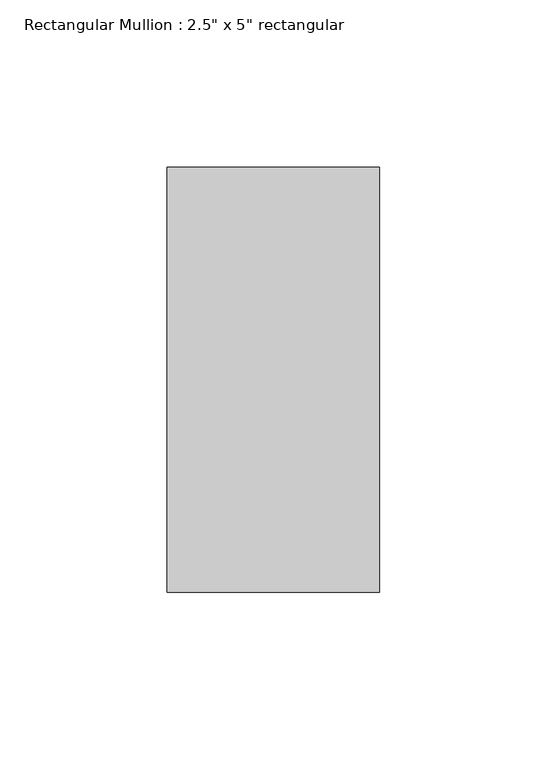
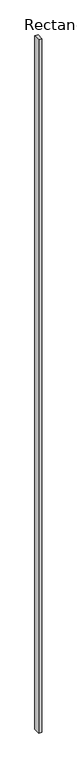
"""IFC4 building model written with IfcOpenShell, lengths in millimetres: member geometry."""

from ifc_helpers import new_model, si_unit, frame, origin, place, context, project, spatial, polyline, outline, extrude, source, transform, mapped, element, save


def member_cf944bc0(model_context):
    return source(origin(), model_context, "Body", "SweptSolid", [
        extrude(outline(polyline([(0.0, 63.5), (0.0, -63.5), (-63.5, -63.5), (-63.5, 63.5), (0.0, 63.5)])), frame((0.0, 0.0, -14630.4), z_axis=(0.0, 0.0, 1.0), x_axis=(1.0, 0.0, 0.0)), (0.0, 0.0, 1.0), 14630.4),
    ])


if __name__ == "__main__":
    model = new_model("IFC4")
    model_context = context("Model", 3, world=origin())
    ifc_project = project(units=[si_unit("LENGTHUNIT", "METRE", prefix="MILLI")], contexts=[model_context])
    site = spatial("IfcSite", under=ifc_project)
    building = spatial("IfcBuilding", under=site)
    placement = place(None, origin())
    member_shape = member_cf944bc0(model_context)
    element("IfcMember", 1, ObjectType="Rectangular Mullion : 2.5\" x 5\" rectangular", at=placement, inside=building, context=model_context, shape_type="MappedRepresentation", body=[
        mapped(member_shape, transform((0.0, 0.0, 0.0), x_axis=(1.0, 0.0, 0.0), y_axis=(0.0, 1.0, 0.0), z_axis=(0.0, 0.0, 1.0))),
    ])
    save(model, "model.ifc")

# Revit data of these elements
# Type "Rectangular Mullion : 2.5\" x 5\" rectangular"
#   built-in parameter 1007304 = 0.416667 (stored number, unit not read)
#   built-in parameter 1007301 = 0.104167 (stored number, unit not read)
#   built-in parameter 1007300 = 0.104167 (stored number, unit not read)
# Element 1 (IfcMember, "Rectangular Mullion : 2.5\" x 5\" rectangular")
#   Materials on its faces: "Aluminum"
# Materials
#   "Aluminum": class "Metal", colour RGB 247 247 247, transparency 0, Description = "Aluminum 6061", Cost = 0
